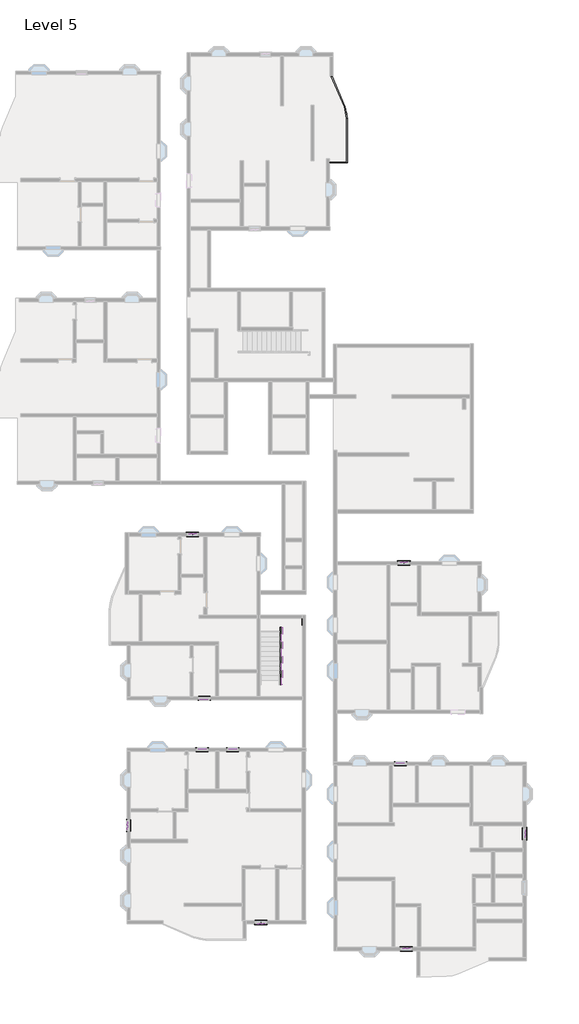
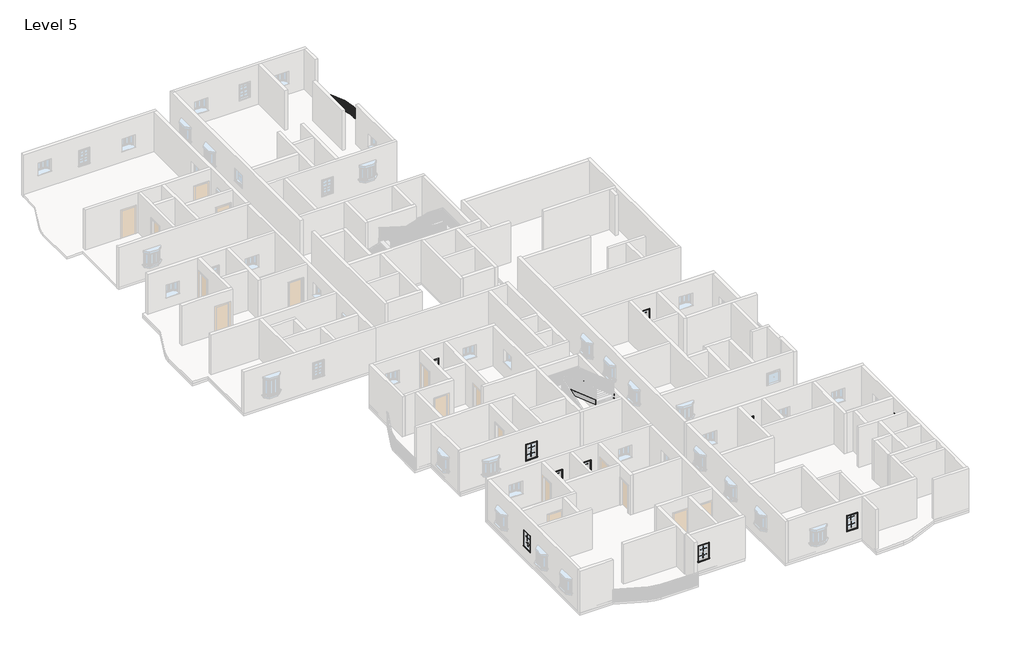
# One storey, part 13 of 14: 40 proxies, 6 members, 1 railing.
"""IFC4 building model written with IfcOpenShell, lengths in millimetres."""

from ifc_helpers import new_model, si_unit, frame, origin, place, context, project, spatial, polyline, circle_curve, outline, extrude, transform, mapped, element, save
from ifc_brep_helpers import plane_surface, cylinder_surface, revolved_surface, advanced_brep
from components import muntin_pattern_2x2_muntin_pattern_2x2_c35c595f, trim_window_exterior_flat_with_sill_e38017c9, trim_window_interior_flat_picture_frame_d728ed12

model = new_model("IFC4")

# Units and contexts
model_context = context("Model", 3, world=origin())
ifc_project = project(units=[si_unit("LENGTHUNIT", "METRE", prefix="MILLI")], contexts=[model_context])

# Site, building, storey
site = spatial("IfcSite", under=ifc_project)
building = spatial("IfcBuilding", under=site)
storey = spatial("IfcBuildingStorey", under=building, Name="Level 5", Elevation=12192.0)

# Proxies
placement = place(None, origin())
muntin_pattern_2x2_muntin_pattern_2x2_shape = muntin_pattern_2x2_muntin_pattern_2x2_c35c595f(model_context)
element("IfcBuildingElementProxy", 1, Name="Muntin Pattern_2x2 : Muntin Pattern_2x2", ObjectType="Muntin Pattern_2x2 : Muntin Pattern_2x2", at=placement, inside=storey, context=model_context, shape_type="MappedRepresentation", body=[
    mapped(muntin_pattern_2x2_muntin_pattern_2x2_shape, transform((-8150.287215, -357.5666506, 13662.025), x_axis=(1.0, 0.0, 0.0), y_axis=(0.0, 1.0, 0.0), z_axis=(0.0, 0.0, 1.0))),
])
element("IfcBuildingElementProxy", 2, Name="Muntin Pattern_2x2 : Muntin Pattern_2x2", ObjectType="Muntin Pattern_2x2 : Muntin Pattern_2x2", at=placement, inside=storey, context=model_context, shape_type="MappedRepresentation", body=[
    mapped(muntin_pattern_2x2_muntin_pattern_2x2_shape, transform((-8150.287215, -402.0166506, 13182.6), x_axis=(1.0, 0.0, 0.0), y_axis=(0.0, 1.0, 0.0), z_axis=(0.0, 0.0, 1.0))),
])
element("IfcBuildingElementProxy", 3, Name="Muntin Pattern_2x2 : Muntin Pattern_2x2", ObjectType="Muntin Pattern_2x2 : Muntin Pattern_2x2", at=placement, inside=storey, context=model_context, shape_type="MappedRepresentation", body=[
    mapped(muntin_pattern_2x2_muntin_pattern_2x2_shape, transform((-7397.812215, -10854.1166506, 13662.025), x_axis=(-1.0, 0.0, 0.0), y_axis=(0.0, -1.0, 0.0), z_axis=(0.0, 0.0, 1.0))),
])
element("IfcBuildingElementProxy", 4, Name="Muntin Pattern_2x2 : Muntin Pattern_2x2", ObjectType="Muntin Pattern_2x2 : Muntin Pattern_2x2", at=placement, inside=storey, context=model_context, shape_type="MappedRepresentation", body=[
    mapped(muntin_pattern_2x2_muntin_pattern_2x2_shape, transform((-7397.812215, -10809.6666506, 13182.6), x_axis=(-1.0, 0.0, 0.0), y_axis=(0.0, -1.0, 0.0), z_axis=(0.0, 0.0, 1.0))),
])
element("IfcBuildingElementProxy", 5, Name="Muntin Pattern_2x2 : Muntin Pattern_2x2", ObjectType="Muntin Pattern_2x2 : Muntin Pattern_2x2", at=placement, inside=storey, context=model_context, shape_type="MappedRepresentation", body=[
    mapped(muntin_pattern_2x2_muntin_pattern_2x2_shape, transform((-7540.687215, -13997.3666506, 13662.025), x_axis=(1.0, 0.0, 0.0), y_axis=(0.0, 1.0, 0.0), z_axis=(0.0, 0.0, 1.0))),
])
element("IfcBuildingElementProxy", 6, Name="Muntin Pattern_2x2 : Muntin Pattern_2x2", ObjectType="Muntin Pattern_2x2 : Muntin Pattern_2x2", at=placement, inside=storey, context=model_context, shape_type="MappedRepresentation", body=[
    mapped(muntin_pattern_2x2_muntin_pattern_2x2_shape, transform((-7540.687215, -14041.8166506, 13182.6), x_axis=(1.0, 0.0, 0.0), y_axis=(0.0, 1.0, 0.0), z_axis=(0.0, 0.0, 1.0))),
])
element("IfcBuildingElementProxy", 7, Name="Muntin Pattern_2x2 : Muntin Pattern_2x2", ObjectType="Muntin Pattern_2x2 : Muntin Pattern_2x2", at=placement, inside=storey, context=model_context, shape_type="MappedRepresentation", body=[
    mapped(muntin_pattern_2x2_muntin_pattern_2x2_shape, transform((-5597.587215, -13997.3666506, 13662.025), x_axis=(1.0, 0.0, 0.0), y_axis=(0.0, 1.0, 0.0), z_axis=(0.0, 0.0, 1.0))),
])
element("IfcBuildingElementProxy", 8, Name="Muntin Pattern_2x2 : Muntin Pattern_2x2", ObjectType="Muntin Pattern_2x2 : Muntin Pattern_2x2", at=placement, inside=storey, context=model_context, shape_type="MappedRepresentation", body=[
    mapped(muntin_pattern_2x2_muntin_pattern_2x2_shape, transform((-5597.587215, -14041.8166506, 13182.6), x_axis=(1.0, 0.0, 0.0), y_axis=(0.0, 1.0, 0.0), z_axis=(0.0, 0.0, 1.0))),
])
element("IfcBuildingElementProxy", 9, Name="Muntin Pattern_2x2 : Muntin Pattern_2x2", ObjectType="Muntin Pattern_2x2 : Muntin Pattern_2x2", at=placement, inside=storey, context=model_context, shape_type="MappedRepresentation", body=[
    mapped(muntin_pattern_2x2_muntin_pattern_2x2_shape, transform((-12255.562215, -18863.6994419, 13662.025), x_axis=(0.0, 1.0, 0.0), y_axis=(-1.0, 0.0, 0.0), z_axis=(0.0, 0.0, 1.0))),
])
element("IfcBuildingElementProxy", 10, Name="Muntin Pattern_2x2 : Muntin Pattern_2x2", ObjectType="Muntin Pattern_2x2 : Muntin Pattern_2x2", at=placement, inside=storey, context=model_context, shape_type="MappedRepresentation", body=[
    mapped(muntin_pattern_2x2_muntin_pattern_2x2_shape, transform((-12211.112215, -18863.6994419, 13182.6), x_axis=(0.0, 1.0, 0.0), y_axis=(-1.0, 0.0, 0.0), z_axis=(0.0, 0.0, 1.0))),
])
element("IfcBuildingElementProxy", 11, Name="Muntin Pattern_2x2 : Muntin Pattern_2x2", ObjectType="Muntin Pattern_2x2 : Muntin Pattern_2x2", at=placement, inside=storey, context=model_context, shape_type="MappedRepresentation", body=[
    mapped(muntin_pattern_2x2_muntin_pattern_2x2_shape, transform((-3806.2891351, -25065.4166506, 13662.025), x_axis=(-1.0, 0.0, 0.0), y_axis=(0.0, -1.0, 0.0), z_axis=(0.0, 0.0, 1.0))),
])
element("IfcBuildingElementProxy", 12, Name="Muntin Pattern_2x2 : Muntin Pattern_2x2", ObjectType="Muntin Pattern_2x2 : Muntin Pattern_2x2", at=placement, inside=storey, context=model_context, shape_type="MappedRepresentation", body=[
    mapped(muntin_pattern_2x2_muntin_pattern_2x2_shape, transform((-3806.2891351, -25020.9666506, 13182.6), x_axis=(-1.0, 0.0, 0.0), y_axis=(0.0, -1.0, 0.0), z_axis=(0.0, 0.0, 1.0))),
])
element("IfcBuildingElementProxy", 13, Name="Muntin Pattern_2x2 : Muntin Pattern_2x2", ObjectType="Muntin Pattern_2x2 : Muntin Pattern_2x2", at=placement, inside=storey, context=model_context, shape_type="MappedRepresentation", body=[
    mapped(muntin_pattern_2x2_muntin_pattern_2x2_shape, transform((5410.0380523, -26615.6292694, 13662.025), x_axis=(1.0, 0.0, 0.0), y_axis=(0.0, 1.0, 0.0), z_axis=(0.0, 0.0, 1.0))),
])
element("IfcBuildingElementProxy", 14, Name="Muntin Pattern_2x2 : Muntin Pattern_2x2", ObjectType="Muntin Pattern_2x2 : Muntin Pattern_2x2", at=placement, inside=storey, context=model_context, shape_type="MappedRepresentation", body=[
    mapped(muntin_pattern_2x2_muntin_pattern_2x2_shape, transform((5410.0380523, -26660.0792694, 13182.6), x_axis=(1.0, 0.0, 0.0), y_axis=(0.0, 1.0, 0.0), z_axis=(0.0, 0.0, 1.0))),
])
element("IfcBuildingElementProxy", 15, Name="Muntin Pattern_2x2 : Muntin Pattern_2x2", ObjectType="Muntin Pattern_2x2 : Muntin Pattern_2x2", at=placement, inside=storey, context=model_context, shape_type="MappedRepresentation", body=[
    mapped(muntin_pattern_2x2_muntin_pattern_2x2_shape, transform((12982.4130523, -19379.8042694, 13662.025), x_axis=(0.0, -1.0, 0.0), y_axis=(1.0, 0.0, 0.0), z_axis=(0.0, 0.0, 1.0))),
])
element("IfcBuildingElementProxy", 16, Name="Muntin Pattern_2x2 : Muntin Pattern_2x2", ObjectType="Muntin Pattern_2x2 : Muntin Pattern_2x2", at=placement, inside=storey, context=model_context, shape_type="MappedRepresentation", body=[
    mapped(muntin_pattern_2x2_muntin_pattern_2x2_shape, transform((12937.9630523, -19379.8042694, 13182.6), x_axis=(0.0, -1.0, 0.0), y_axis=(1.0, 0.0, 0.0), z_axis=(0.0, 0.0, 1.0))),
])
element("IfcBuildingElementProxy", 17, Name="Muntin Pattern_2x2 : Muntin Pattern_2x2", ObjectType="Muntin Pattern_2x2 : Muntin Pattern_2x2", at=placement, inside=storey, context=model_context, shape_type="MappedRepresentation", body=[
    mapped(muntin_pattern_2x2_muntin_pattern_2x2_shape, transform((5048.0880523, -14880.8292694, 13662.025), x_axis=(1.0, 0.0, 0.0), y_axis=(0.0, 1.0, 0.0), z_axis=(0.0, 0.0, 1.0))),
])
element("IfcBuildingElementProxy", 18, Name="Muntin Pattern_2x2 : Muntin Pattern_2x2", ObjectType="Muntin Pattern_2x2 : Muntin Pattern_2x2", at=placement, inside=storey, context=model_context, shape_type="MappedRepresentation", body=[
    mapped(muntin_pattern_2x2_muntin_pattern_2x2_shape, transform((5048.0880523, -14925.2792694, 13182.6), x_axis=(1.0, 0.0, 0.0), y_axis=(0.0, 1.0, 0.0), z_axis=(0.0, 0.0, 1.0))),
])
element("IfcBuildingElementProxy", 19, Name="Muntin Pattern_2x2 : Muntin Pattern_2x2", ObjectType="Muntin Pattern_2x2 : Muntin Pattern_2x2", at=placement, inside=storey, context=model_context, shape_type="MappedRepresentation", body=[
    mapped(muntin_pattern_2x2_muntin_pattern_2x2_shape, transform((5257.6380523, -2168.1292694, 13662.025), x_axis=(1.0, 0.0, 0.0), y_axis=(0.0, 1.0, 0.0), z_axis=(0.0, 0.0, 1.0))),
])
element("IfcBuildingElementProxy", 20, Name="Muntin Pattern_2x2 : Muntin Pattern_2x2", ObjectType="Muntin Pattern_2x2 : Muntin Pattern_2x2", at=placement, inside=storey, context=model_context, shape_type="MappedRepresentation", body=[
    mapped(muntin_pattern_2x2_muntin_pattern_2x2_shape, transform((5257.6380523, -2212.5792694, 13182.6), x_axis=(1.0, 0.0, 0.0), y_axis=(0.0, 1.0, 0.0), z_axis=(0.0, 0.0, 1.0))),
])
trim_window_exterior_flat_with_sill_shape = trim_window_exterior_flat_with_sill_e38017c9(model_context)
element("IfcBuildingElementProxy", 21, Name="Trim-Window-Exterior-Flat : with Sill", ObjectType="Trim-Window-Exterior-Flat : with Sill", at=placement, inside=storey, context=model_context, shape_type="MappedRepresentation", body=[
    mapped(trim_window_exterior_flat_with_sill_shape, transform((-8150.287215, -322.6416506, 14173.2), x_axis=(-1.0, 0.0, 0.0), y_axis=(0.0, 0.0, 1.0), z_axis=(0.0, 1.0, 0.0))),
])
element("IfcBuildingElementProxy", 22, Name="Trim-Window-Exterior-Flat : with Sill", ObjectType="Trim-Window-Exterior-Flat : with Sill", at=placement, inside=storey, context=model_context, shape_type="MappedRepresentation", body=[
    mapped(trim_window_exterior_flat_with_sill_shape, transform((-7397.812215, -10889.0416506, 14173.2), x_axis=(1.0, 0.0, 0.0), y_axis=(0.0, 0.0, 1.0), z_axis=(0.0, -1.0, 0.0))),
])
element("IfcBuildingElementProxy", 23, Name="Trim-Window-Exterior-Flat : with Sill", ObjectType="Trim-Window-Exterior-Flat : with Sill", at=placement, inside=storey, context=model_context, shape_type="MappedRepresentation", body=[
    mapped(trim_window_exterior_flat_with_sill_shape, transform((-7540.687215, -13962.4416506, 14173.2), x_axis=(-1.0, 0.0, 0.0), y_axis=(0.0, 0.0, 1.0), z_axis=(0.0, 1.0, 0.0))),
])
element("IfcBuildingElementProxy", 24, Name="Trim-Window-Exterior-Flat : with Sill", ObjectType="Trim-Window-Exterior-Flat : with Sill", at=placement, inside=storey, context=model_context, shape_type="MappedRepresentation", body=[
    mapped(trim_window_exterior_flat_with_sill_shape, transform((-5597.587215, -13962.4416506, 14173.2), x_axis=(-1.0, 0.0, 0.0), y_axis=(0.0, 0.0, 1.0), z_axis=(0.0, 1.0, 0.0))),
])
element("IfcBuildingElementProxy", 25, Name="Trim-Window-Exterior-Flat : with Sill", ObjectType="Trim-Window-Exterior-Flat : with Sill", at=placement, inside=storey, context=model_context, shape_type="MappedRepresentation", body=[
    mapped(trim_window_exterior_flat_with_sill_shape, transform((-12290.487215, -18863.6994419, 14173.2), x_axis=(0.0, -1.0, 0.0), y_axis=(0.0, 0.0, 1.0), z_axis=(-1.0, 0.0, 0.0))),
])
element("IfcBuildingElementProxy", 26, Name="Trim-Window-Exterior-Flat : with Sill", ObjectType="Trim-Window-Exterior-Flat : with Sill", at=placement, inside=storey, context=model_context, shape_type="MappedRepresentation", body=[
    mapped(trim_window_exterior_flat_with_sill_shape, transform((-3806.2891351, -25100.3416506, 14173.2), x_axis=(1.0, 0.0, 0.0), y_axis=(0.0, 0.0, 1.0), z_axis=(0.0, -1.0, 0.0))),
])
element("IfcBuildingElementProxy", 27, Name="Trim-Window-Exterior-Flat : with Sill", ObjectType="Trim-Window-Exterior-Flat : with Sill", at=placement, inside=storey, context=model_context, shape_type="MappedRepresentation", body=[
    mapped(trim_window_exterior_flat_with_sill_shape, transform((5410.0380523, -26580.7042694, 14173.2), x_axis=(-1.0, 0.0, 0.0), y_axis=(0.0, 0.0, 1.0), z_axis=(0.0, 1.0, 0.0))),
])
element("IfcBuildingElementProxy", 28, Name="Trim-Window-Exterior-Flat : with Sill", ObjectType="Trim-Window-Exterior-Flat : with Sill", at=placement, inside=storey, context=model_context, shape_type="MappedRepresentation", body=[
    mapped(trim_window_exterior_flat_with_sill_shape, transform((13017.3380523, -19379.8042694, 14173.2), x_axis=(0.0, 1.0, 0.0), y_axis=(0.0, 0.0, 1.0), z_axis=(1.0, 0.0, 0.0))),
])
element("IfcBuildingElementProxy", 29, Name="Trim-Window-Exterior-Flat : with Sill", ObjectType="Trim-Window-Exterior-Flat : with Sill", at=placement, inside=storey, context=model_context, shape_type="MappedRepresentation", body=[
    mapped(trim_window_exterior_flat_with_sill_shape, transform((5048.0880523, -14845.9042694, 14173.2), x_axis=(-1.0, 0.0, 0.0), y_axis=(0.0, 0.0, 1.0), z_axis=(0.0, 1.0, 0.0))),
])
element("IfcBuildingElementProxy", 30, Name="Trim-Window-Exterior-Flat : with Sill", ObjectType="Trim-Window-Exterior-Flat : with Sill", at=placement, inside=storey, context=model_context, shape_type="MappedRepresentation", body=[
    mapped(trim_window_exterior_flat_with_sill_shape, transform((5257.6380523, -2133.2042694, 14173.2), x_axis=(-1.0, 0.0, 0.0), y_axis=(0.0, 0.0, 1.0), z_axis=(0.0, 1.0, 0.0))),
])
trim_window_interior_flat_picture_frame_shape = trim_window_interior_flat_picture_frame_d728ed12(model_context)
element("IfcBuildingElementProxy", 31, Name="Trim-Window-Interior-Flat : Picture Frame", ObjectType="Trim-Window-Interior-Flat : Picture Frame", at=placement, inside=storey, context=model_context, shape_type="MappedRepresentation", body=[
    mapped(trim_window_interior_flat_picture_frame_shape, transform((-8150.287215, -525.8416506, 14173.2), x_axis=(1.0, 0.0, 0.0), y_axis=(0.0, 0.0, 1.0), z_axis=(0.0, -1.0, 0.0))),
])
element("IfcBuildingElementProxy", 32, Name="Trim-Window-Interior-Flat : Picture Frame", ObjectType="Trim-Window-Interior-Flat : Picture Frame", at=placement, inside=storey, context=model_context, shape_type="MappedRepresentation", body=[
    mapped(trim_window_interior_flat_picture_frame_shape, transform((-7397.812215, -10685.8416506, 14173.2), x_axis=(-1.0, 0.0, 0.0), y_axis=(0.0, 0.0, 1.0), z_axis=(0.0, 1.0, 0.0))),
])
element("IfcBuildingElementProxy", 33, Name="Trim-Window-Interior-Flat : Picture Frame", ObjectType="Trim-Window-Interior-Flat : Picture Frame", at=placement, inside=storey, context=model_context, shape_type="MappedRepresentation", body=[
    mapped(trim_window_interior_flat_picture_frame_shape, transform((-7540.687215, -14165.6416506, 14173.2), x_axis=(1.0, 0.0, 0.0), y_axis=(0.0, 0.0, 1.0), z_axis=(0.0, -1.0, 0.0))),
])
element("IfcBuildingElementProxy", 34, Name="Trim-Window-Interior-Flat : Picture Frame", ObjectType="Trim-Window-Interior-Flat : Picture Frame", at=placement, inside=storey, context=model_context, shape_type="MappedRepresentation", body=[
    mapped(trim_window_interior_flat_picture_frame_shape, transform((-5597.587215, -14165.6416506, 14173.2), x_axis=(1.0, 0.0, 0.0), y_axis=(0.0, 0.0, 1.0), z_axis=(0.0, -1.0, 0.0))),
])
element("IfcBuildingElementProxy", 35, Name="Trim-Window-Interior-Flat : Picture Frame", ObjectType="Trim-Window-Interior-Flat : Picture Frame", at=placement, inside=storey, context=model_context, shape_type="MappedRepresentation", body=[
    mapped(trim_window_interior_flat_picture_frame_shape, transform((-12087.287215, -18863.6994419, 14173.2), x_axis=(0.0, 1.0, 0.0), y_axis=(0.0, 0.0, 1.0), z_axis=(1.0, 0.0, 0.0))),
])
element("IfcBuildingElementProxy", 36, Name="Trim-Window-Interior-Flat : Picture Frame", ObjectType="Trim-Window-Interior-Flat : Picture Frame", at=placement, inside=storey, context=model_context, shape_type="MappedRepresentation", body=[
    mapped(trim_window_interior_flat_picture_frame_shape, transform((-3806.2891351, -24897.1416506, 14173.2), x_axis=(-1.0, 0.0, 0.0), y_axis=(0.0, 0.0, 1.0), z_axis=(0.0, 1.0, 0.0))),
])
element("IfcBuildingElementProxy", 37, Name="Trim-Window-Interior-Flat : Picture Frame", ObjectType="Trim-Window-Interior-Flat : Picture Frame", at=placement, inside=storey, context=model_context, shape_type="MappedRepresentation", body=[
    mapped(trim_window_interior_flat_picture_frame_shape, transform((5410.0380523, -26783.9042694, 14173.2), x_axis=(1.0, 0.0, 0.0), y_axis=(0.0, 0.0, 1.0), z_axis=(0.0, -1.0, 0.0))),
])
element("IfcBuildingElementProxy", 38, Name="Trim-Window-Interior-Flat : Picture Frame", ObjectType="Trim-Window-Interior-Flat : Picture Frame", at=placement, inside=storey, context=model_context, shape_type="MappedRepresentation", body=[
    mapped(trim_window_interior_flat_picture_frame_shape, transform((12814.1380523, -19379.8042694, 14173.2), x_axis=(0.0, -1.0, 0.0), y_axis=(0.0, 0.0, 1.0), z_axis=(-1.0, 0.0, 0.0))),
])
element("IfcBuildingElementProxy", 39, Name="Trim-Window-Interior-Flat : Picture Frame", ObjectType="Trim-Window-Interior-Flat : Picture Frame", at=placement, inside=storey, context=model_context, shape_type="MappedRepresentation", body=[
    mapped(trim_window_interior_flat_picture_frame_shape, transform((5048.0880523, -15049.1042694, 14173.2), x_axis=(1.0, 0.0, 0.0), y_axis=(0.0, 0.0, 1.0), z_axis=(0.0, -1.0, 0.0))),
])
element("IfcBuildingElementProxy", 40, Name="Trim-Window-Interior-Flat : Picture Frame", ObjectType="Trim-Window-Interior-Flat : Picture Frame", at=placement, inside=storey, context=model_context, shape_type="MappedRepresentation", body=[
    mapped(trim_window_interior_flat_picture_frame_shape, transform((5257.6380523, -2336.4042694, 14173.2), x_axis=(1.0, 0.0, 0.0), y_axis=(0.0, 0.0, 1.0), z_axis=(0.0, -1.0, 0.0))),
])

# Members
element("IfcMember", 41, ObjectType="Stringer - 2\" Width", at=placement, inside=storey, context=model_context, shape_type="SweptSolid", body=[
    extrude(outline(polyline([(-9955.5916506, 12192.0), (-9955.5916506, 12383.3592169), (-6325.8738327, 13639.8), (-5713.7916506, 13639.8), (-5713.7916506, 13529.1301656), (-9576.612129, 12192.0), (-9955.5916506, 12192.0)])), frame((-3908.487215, 0.0, 0.0), z_axis=(1.0, 0.0, 0.0), x_axis=(0.0, 1.0, 0.0)), (0.0, 0.0, 1.0), 50.8),
])
element("IfcMember", 42, ObjectType="Stringer - 2\" Width", at=placement, inside=storey, context=model_context, shape_type="SweptSolid", body=[
    extrude(outline(polyline([(-3908.487215, -5713.7916506), (-3908.487215, -5662.9916506), (-1190.687215, -5662.9916506), (-1190.687215, -5713.7916506), (-3908.487215, -5713.7916506)])), frame((0.0, 0.0, 13335.0), z_axis=(0.0, 0.0, 1.0), x_axis=(1.0, 0.0, 0.0)), (0.0, 0.0, 1.0), 304.8),
])
element("IfcMember", 43, ObjectType="Stringer - 2\" Width", at=placement, inside=storey, context=model_context, shape_type="SweptSolid", body=[
    extrude(outline(polyline([(-5662.9916506, 13539.5476784), (-5662.9916506, 13335.0), (-6003.8711722, 13335.0), (-9949.2416506, 14700.7051656), (-9949.2416506, 15023.2496015), (-5662.9916506, 13539.5476784)])), frame((-1190.687215, 0.0, 0.0), z_axis=(1.0, 0.0, 0.0), x_axis=(0.0, 1.0, 0.0)), (0.0, 0.0, 1.0), 50.8),
])
element("IfcMember", 44, ObjectType="Stringer - 2\" Width", at=placement, inside=storey, context=model_context, shape_type="SweptSolid", body=[
    extrude(outline(polyline([(-9955.5916506, 12192.0), (-9955.5916506, 12383.3592169), (-6342.4416506, 13634.0649861), (-6342.4416506, 13311.5205502), (-9576.612129, 12192.0), (-9955.5916506, 12192.0)])), frame((-2593.7381751, 0.0, 0.0), z_axis=(1.0, 0.0, 0.0), x_axis=(0.0, 1.0, 0.0)), (0.0, 0.0, 1.0), 50.8),
])
element("IfcMember", 45, ObjectType="Stringer - 2\" Width", at=placement, inside=storey, context=model_context, shape_type="SweptSolid", body=[
    extrude(outline(polyline([(-2593.7381751, -6342.4416506), (-2593.7381751, -6291.6416506), (-2492.1381751, -6291.6416506), (-2492.1381751, -6342.4416506), (-2593.7381751, -6342.4416506)])), frame((0.0, 0.0, 13335.0), z_axis=(0.0, 0.0, 1.0), x_axis=(1.0, 0.0, 0.0)), (0.0, 0.0, 1.0), 304.8),
])
element("IfcMember", 46, ObjectType="Stringer - 2\" Width", at=placement, inside=storey, context=model_context, shape_type="SweptSolid", body=[
    extrude(outline(polyline([(-6291.6416506, 13757.1572938), (-6291.6416506, 13434.6128579), (-9949.2416506, 14700.7051656), (-9949.2416506, 15023.2496015), (-6291.6416506, 13757.1572938)])), frame((-2492.1381751, 0.0, 0.0), z_axis=(1.0, 0.0, 0.0), x_axis=(0.0, 1.0, 0.0)), (0.0, 0.0, 1.0), 50.8),
])

# Railing
element("IfcRailing", 47, ObjectType="Handrail - Rectangular", at=placement, inside=storey, context=model_context, shape_type="SolidModel", body=[
    advanced_brep(
    [(549.8108649, 23180.4215905, 13106.4), (549.8108649, 23180.4215905, 13055.6), (549.8108649, 23129.6215905, 13055.6), (549.8108649, 23129.6215905, 13106.4), (1629.3108649, 23180.4215905, 13106.4), (1629.3108649, 23180.4215905, 13055.6), (1680.1108649, 23129.6215905, 13055.6), (1680.1108649, 23129.6215905, 13106.4), (1629.3108649, 25921.9580583, 13106.4), (1629.3108649, 25921.9580583, 13055.6), (1680.1108649, 25921.9580583, 13055.6), (1680.1108649, 25921.9580583, 13106.4), (1475.5051478, 26671.8537734, 13055.6), (1475.5051478, 26671.8537734, 13106.4), (1522.203662, 26691.8509925, 13055.6), (1522.203662, 26691.8509925, 13106.4), (640.7616078, 28621.188975, 13106.4), (687.460122, 28641.186194, 13106.4), (687.460122, 28641.186194, 13055.6), (640.7616078, 28621.188975, 13055.6)],
    [
        (0, 1),
        (1, 2),
        (2, 3),
        (3, 0),
        (0, 4),
        (4, 5),
        (5, 1),
        (5, 6),
        (6, 2),
        (6, 7),
        (7, 3),
        (7, 4),
        (4, 8),
        (8, 9),
        (9, 5),
        (9, 10),
        (10, 6),
        (10, 11),
        (11, 7),
        (11, 8),
        (12, 9, circle_curve(frame((-275.6891351, 25921.9580583, 13055.6), z_axis=(0.0, 0.0, -1.0), x_axis=(1.0, 0.0, 0.0)), 1905.0)),
        (8, 13, circle_curve(frame((-275.6891351, 25921.9580583, 13106.4), z_axis=(0.0, 0.0, 1.0), x_axis=(1.0, 0.0, 0.0)), 1905.0)),
        (13, 12),
        (14, 10, circle_curve(frame((-275.6891351, 25921.9580583, 13055.6), z_axis=(0.0, 0.0, -1.0), x_axis=(1.0, 0.0, 0.0)), 1955.8)),
        (12, 14),
        (15, 11, circle_curve(frame((-275.6891351, 25921.9580583, 13106.4), z_axis=(0.0, 0.0, -1.0), x_axis=(1.0, 0.0, 0.0)), 1955.8)),
        (14, 15),
        (15, 13),
        (16, 17),
        (17, 18),
        (18, 19),
        (19, 16),
        (13, 16),
        (19, 12),
        (18, 14),
        (17, 15),
    ],
    [
        plane_surface(frame((549.8108649, 23155.0215905, 13106.4), z_axis=(-1.0, 0.0, 0.0), x_axis=(0.0, 1.0, 0.0))),
        plane_surface(frame((549.8108649, 23180.4215905, 13106.4), z_axis=(0.0, 1.0, 0.0), x_axis=(1.0, 0.0, 0.0))),
        plane_surface(frame((549.8108649, 23180.4215905, 13055.6), z_axis=(0.0, 0.0, -1.0), x_axis=(1.0, 0.0, 0.0))),
        plane_surface(frame((549.8108649, 23129.6215905, 13055.6), z_axis=(0.0, -1.0, 0.0), x_axis=(1.0, 0.0, 0.0))),
        plane_surface(frame((549.8108649, 23129.6215905, 13106.4), z_axis=(0.0, 0.0, 1.0), x_axis=(1.0, 0.0, 0.0))),
        plane_surface(frame((1629.3108649, 23180.4215905, 13106.4), z_axis=(-1.0, 0.0, 0.0), x_axis=(0.0, 1.0, 0.0))),
        plane_surface(frame((1629.3108649, 23180.4215905, 13055.6), z_axis=(0.0, 0.0, -1.0), x_axis=(0.0, 1.0, 0.0))),
        plane_surface(frame((1680.1108649, 23129.6215905, 13055.6), z_axis=(1.0, 0.0, 0.0), x_axis=(0.0, 1.0, 0.0))),
        plane_surface(frame((1680.1108649, 23129.6215905, 13106.4), z_axis=(0.0, 0.0, 1.0), x_axis=(0.0, 1.0, 0.0))),
        revolved_surface(polyline([(1629.3108649, 25921.9580583, 13106.4), (1629.3108649, 25921.9580583, 13055.6)]), (-275.6891351, 25921.9580583, 13106.4), (0.0, 0.0, 1.0)),
        plane_surface(frame((-275.6891351, 25921.9580583, 13055.6), z_axis=(0.0, 0.0, -1.0), x_axis=(1.0, 0.0, 0.0))),
        cylinder_surface(frame((-275.6891351, 25921.9580583, 13106.4), z_axis=(0.0, 0.0, 1.0), x_axis=(1.0, 0.0, 0.0)), 1955.8),
        plane_surface(frame((-275.6891351, 25921.9580583, 13106.4), z_axis=(0.0, 0.0, 1.0), x_axis=(1.0, 0.0, 0.0))),
        plane_surface(frame((664.1108649, 28631.1875845, 13106.4), z_axis=(-0.39364604467361036, 0.91926209076238, 0.0), x_axis=(0.91926209076238, 0.39364604467361036, 0.0))),
        plane_surface(frame((1475.5051478, 26671.8537734, 13106.4), z_axis=(-0.91926209076238, -0.3936460446736102, 0.0), x_axis=(-0.3936460446736102, 0.91926209076238, 0.0))),
        plane_surface(frame((1475.5051478, 26671.8537734, 13055.6), z_axis=(0.0, 0.0, -1.0), x_axis=(-0.3936460446736102, 0.91926209076238, 0.0))),
        plane_surface(frame((1522.203662, 26691.8509925, 13055.6), z_axis=(0.91926209076238, 0.3936460446736102, 0.0), x_axis=(-0.3936460446736102, 0.91926209076238, 0.0))),
        plane_surface(frame((1522.203662, 26691.8509925, 13106.4), z_axis=(0.0, 0.0, 1.0), x_axis=(-0.3936460446736102, 0.91926209076238, 0.0))),
    ],
    [
        (0, [[1, 2, 3, 4]]),
        (1, [[-1, 5, 6, 7]]),
        (2, [[-2, -7, 8, 9]]),
        (3, [[-3, -9, 10, 11]]),
        (4, [[-4, -11, 12, -5]]),
        (5, [[-6, 13, 14, 15]]),
        (6, [[-8, -15, 16, 17]]),
        (7, [[-10, -17, 18, 19]]),
        (8, [[-12, -19, 20, -13]]),
        (9, [[21, -14, 22, 23]]),
        (10, [[24, -16, -21, 25]]),
        (11, [[26, -18, -24, 27]]),
        (12, [[-22, -20, -26, 28]]),
        (13, [[29, 30, 31, 32]]),
        (14, [[-23, 33, -32, 34]]),
        (15, [[-25, -34, -31, 35]]),
        (16, [[-27, -35, -30, 36]]),
        (17, [[-28, -36, -29, -33]]),
    ],
),
    extrude(outline(polyline([(711.4710921, 28544.7864585), (693.9591493, 28537.2875014), (686.4601921, 28554.7994442), (703.9721349, 28562.2984014), (711.4710921, 28544.7864585)])), frame((0.0, 0.0, 12192.0), z_axis=(0.0, 0.0, 1.0), x_axis=(1.0, 0.0, 0.0)), (0.0, 0.0, 1.0), 863.6),
    extrude(outline(polyline([(751.4655302, 28451.3894301), (733.9535874, 28443.890473), (726.4546303, 28461.4024158), (743.9665731, 28468.9013729), (751.4655302, 28451.3894301)])), frame((0.0, 0.0, 12192.0), z_axis=(0.0, 0.0, 1.0), x_axis=(1.0, 0.0, 0.0)), (0.0, 0.0, 1.0), 863.6),
    extrude(outline(polyline([(791.4599684, 28357.9924017), (773.9480255, 28350.4934445), (766.4490684, 28368.0053874), (783.9610112, 28375.5043445), (791.4599684, 28357.9924017)])), frame((0.0, 0.0, 12192.0), z_axis=(0.0, 0.0, 1.0), x_axis=(1.0, 0.0, 0.0)), (0.0, 0.0, 1.0), 863.6),
    extrude(outline(polyline([(831.4544065, 28264.5953733), (813.9424637, 28257.0964161), (806.4435065, 28274.608359), (823.9554494, 28282.1073161), (831.4544065, 28264.5953733)])), frame((0.0, 0.0, 12192.0), z_axis=(0.0, 0.0, 1.0), x_axis=(1.0, 0.0, 0.0)), (0.0, 0.0, 1.0), 863.6),
    extrude(outline(polyline([(871.4488446, 28171.1983449), (853.9369018, 28163.6993877), (846.4379447, 28181.2113305), (863.9498875, 28188.7102877), (871.4488446, 28171.1983449)])), frame((0.0, 0.0, 12192.0), z_axis=(0.0, 0.0, 1.0), x_axis=(1.0, 0.0, 0.0)), (0.0, 0.0, 1.0), 863.6),
    extrude(outline(polyline([(911.4432828, 28077.8013164), (893.93134, 28070.3023593), (886.4323828, 28087.8143021), (903.9443256, 28095.3132593), (911.4432828, 28077.8013164)])), frame((0.0, 0.0, 12192.0), z_axis=(0.0, 0.0, 1.0), x_axis=(1.0, 0.0, 0.0)), (0.0, 0.0, 1.0), 863.6),
    extrude(outline(polyline([(951.4377209, 27984.404288), (933.9257781, 27976.9053309), (926.4268209, 27994.4172737), (943.9387638, 28001.9162308), (951.4377209, 27984.404288)])), frame((0.0, 0.0, 12192.0), z_axis=(0.0, 0.0, 1.0), x_axis=(1.0, 0.0, 0.0)), (0.0, 0.0, 1.0), 863.6),
    extrude(outline(polyline([(991.4321591, 27891.0072596), (973.9202162, 27883.5083024), (966.4212591, 27901.0202453), (983.9332019, 27908.5192024), (991.4321591, 27891.0072596)])), frame((0.0, 0.0, 12192.0), z_axis=(0.0, 0.0, 1.0), x_axis=(1.0, 0.0, 0.0)), (0.0, 0.0, 1.0), 863.6),
    extrude(outline(polyline([(1031.4265972, 27797.6102312), (1013.9146544, 27790.111274), (1006.4156972, 27807.6232168), (1023.9276401, 27815.122174), (1031.4265972, 27797.6102312)])), frame((0.0, 0.0, 12192.0), z_axis=(0.0, 0.0, 1.0), x_axis=(1.0, 0.0, 0.0)), (0.0, 0.0, 1.0), 863.6),
    extrude(outline(polyline([(1071.4210353, 27704.2132027), (1053.9090925, 27696.7142456), (1046.4101354, 27714.2261884), (1063.9220782, 27721.7251456), (1071.4210353, 27704.2132027)])), frame((0.0, 0.0, 12192.0), z_axis=(0.0, 0.0, 1.0), x_axis=(1.0, 0.0, 0.0)), (0.0, 0.0, 1.0), 863.6),
    extrude(outline(polyline([(1111.4154735, 27610.8161743), (1093.9035307, 27603.3172172), (1086.4045735, 27620.82916), (1103.9165163, 27628.3281172), (1111.4154735, 27610.8161743)])), frame((0.0, 0.0, 12192.0), z_axis=(0.0, 0.0, 1.0), x_axis=(1.0, 0.0, 0.0)), (0.0, 0.0, 1.0), 863.6),
    extrude(outline(polyline([(1151.4099116, 27517.4191459), (1133.8979688, 27509.9201888), (1126.3990116, 27527.4321316), (1143.9109545, 27534.9310887), (1151.4099116, 27517.4191459)])), frame((0.0, 0.0, 12192.0), z_axis=(0.0, 0.0, 1.0), x_axis=(1.0, 0.0, 0.0)), (0.0, 0.0, 1.0), 863.6),
    extrude(outline(polyline([(1191.4043498, 27424.0221175), (1173.8924069, 27416.5231603), (1166.3934498, 27434.0351032), (1183.9053926, 27441.5340603), (1191.4043498, 27424.0221175)])), frame((0.0, 0.0, 12192.0), z_axis=(0.0, 0.0, 1.0), x_axis=(1.0, 0.0, 0.0)), (0.0, 0.0, 1.0), 863.6),
    extrude(outline(polyline([(1231.3987879, 27330.6250891), (1213.8868451, 27323.1261319), (1206.3878879, 27340.6380747), (1223.8998307, 27348.1370319), (1231.3987879, 27330.6250891)])), frame((0.0, 0.0, 12192.0), z_axis=(0.0, 0.0, 1.0), x_axis=(1.0, 0.0, 0.0)), (0.0, 0.0, 1.0), 863.6),
    extrude(outline(polyline([(1271.393226, 27237.2280606), (1253.8812832, 27229.7291035), (1246.3823261, 27247.2410463), (1263.8942689, 27254.7400035), (1271.393226, 27237.2280606)])), frame((0.0, 0.0, 12192.0), z_axis=(0.0, 0.0, 1.0), x_axis=(1.0, 0.0, 0.0)), (0.0, 0.0, 1.0), 863.6),
    extrude(outline(polyline([(1311.3876642, 27143.8310322), (1293.8757213, 27136.3320751), (1286.3767642, 27153.8440179), (1303.888707, 27161.342975), (1311.3876642, 27143.8310322)])), frame((0.0, 0.0, 12192.0), z_axis=(0.0, 0.0, 1.0), x_axis=(1.0, 0.0, 0.0)), (0.0, 0.0, 1.0), 863.6),
    extrude(outline(polyline([(1351.3821023, 27050.4340038), (1333.8701595, 27042.9350466), (1326.3712023, 27060.4469895), (1343.8831452, 27067.9459466), (1351.3821023, 27050.4340038)])), frame((0.0, 0.0, 12192.0), z_axis=(0.0, 0.0, 1.0), x_axis=(1.0, 0.0, 0.0)), (0.0, 0.0, 1.0), 863.6),
    extrude(outline(polyline([(1391.3765405, 26957.0369754), (1373.8645976, 26949.5380182), (1366.3656405, 26967.0499611), (1383.8775833, 26974.5489182), (1391.3765405, 26957.0369754)])), frame((0.0, 0.0, 12192.0), z_axis=(0.0, 0.0, 1.0), x_axis=(1.0, 0.0, 0.0)), (0.0, 0.0, 1.0), 863.6),
    extrude(outline(polyline([(1431.3709786, 26863.639947), (1413.8590358, 26856.1409898), (1406.3600786, 26873.6529326), (1423.8720214, 26881.1518898), (1431.3709786, 26863.639947)])), frame((0.0, 0.0, 12192.0), z_axis=(0.0, 0.0, 1.0), x_axis=(1.0, 0.0, 0.0)), (0.0, 0.0, 1.0), 863.6),
    extrude(outline(polyline([(1471.3654167, 26770.2429185), (1453.8534739, 26762.7439614), (1446.3545168, 26780.2559042), (1463.8664596, 26787.7548614), (1471.3654167, 26770.2429185)])), frame((0.0, 0.0, 12192.0), z_axis=(0.0, 0.0, 1.0), x_axis=(1.0, 0.0, 0.0)), (0.0, 0.0, 1.0), 863.6),
    extrude(outline(polyline([(1537.4917391, 26611.722401), (1519.7200483, 26604.8616791), (1512.8593263, 26622.6333699), (1530.6310171, 26629.4940918), (1537.4917391, 26611.722401)])), frame((0.0, 0.0, 12192.0), z_axis=(0.0, 0.0, 1.0), x_axis=(1.0, 0.0, 0.0)), (0.0, 0.0, 1.0), 863.6),
    extrude(outline(polyline([(1571.2676162, 26515.3807493), (1553.1596103, 26509.4644479), (1547.2433088, 26527.5724538), (1565.3513147, 26533.4887552), (1571.2676162, 26515.3807493)])), frame((0.0, 0.0, 12192.0), z_axis=(0.0, 0.0, 1.0), x_axis=(1.0, 0.0, 0.0)), (0.0, 0.0, 1.0), 863.6),
    extrude(outline(polyline([(1599.9284504, 26417.3956468), (1581.5342785, 26412.4401508), (1576.5787825, 26430.8343227), (1594.9729544, 26435.7898187), (1599.9284504, 26417.3956468)])), frame((0.0, 0.0, 12192.0), z_axis=(0.0, 0.0, 1.0), x_axis=(1.0, 0.0, 0.0)), (0.0, 0.0, 1.0), 863.6),
    extrude(outline(polyline([(1623.3948673, 26318.0384578), (1604.7654711, 26314.0574912), (1600.7845045, 26332.6868874), (1619.4139008, 26336.667854), (1623.3948673, 26318.0384578)])), frame((0.0, 0.0, 12192.0), z_axis=(0.0, 0.0, 1.0), x_axis=(1.0, 0.0, 0.0)), (0.0, 0.0, 1.0), 863.6),
    extrude(outline(polyline([(1641.601878, 26217.5843464), (1622.7888504, 26214.5889343), (1619.7934383, 26233.4019618), (1638.6064659, 26236.3973739), (1641.601878, 26217.5843464)])), frame((0.0, 0.0, 12192.0), z_axis=(0.0, 0.0, 1.0), x_axis=(1.0, 0.0, 0.0)), (0.0, 0.0, 1.0), 863.6),
    extrude(outline(polyline([(1654.4990591, 26116.3115146), (1635.5545019, 26114.3099526), (1633.5529398, 26133.2545098), (1652.4974971, 26135.2560719), (1654.4990591, 26116.3115146)])), frame((0.0, 0.0, 12192.0), z_axis=(0.0, 0.0, 1.0), x_axis=(1.0, 0.0, 0.0)), (0.0, 0.0, 1.0), 863.6),
    extrude(outline(polyline([(1662.0506927, 26014.5004319), (1643.0270716, 26013.4982632), (1642.0249029, 26032.5218842), (1661.048524, 26033.524053), (1662.0506927, 26014.5004319)])), frame((0.0, 0.0, 12192.0), z_axis=(0.0, 0.0, 1.0), x_axis=(1.0, 0.0, 0.0)), (0.0, 0.0, 1.0), 863.6),
    extrude(outline(polyline([(1664.2358649, 25888.6965905), (1645.1858649, 25888.6965905), (1645.1858649, 25907.7465905), (1664.2358649, 25907.7465905), (1664.2358649, 25888.6965905)])), frame((0.0, 0.0, 12192.0), z_axis=(0.0, 0.0, 1.0), x_axis=(1.0, 0.0, 0.0)), (0.0, 0.0, 1.0), 863.6),
    extrude(outline(polyline([(1664.2358649, 25787.0965905), (1645.1858649, 25787.0965905), (1645.1858649, 25806.1465905), (1664.2358649, 25806.1465905), (1664.2358649, 25787.0965905)])), frame((0.0, 0.0, 12192.0), z_axis=(0.0, 0.0, 1.0), x_axis=(1.0, 0.0, 0.0)), (0.0, 0.0, 1.0), 863.6),
    extrude(outline(polyline([(1664.2358649, 25685.4965905), (1645.1858649, 25685.4965905), (1645.1858649, 25704.5465905), (1664.2358649, 25704.5465905), (1664.2358649, 25685.4965905)])), frame((0.0, 0.0, 12192.0), z_axis=(0.0, 0.0, 1.0), x_axis=(1.0, 0.0, 0.0)), (0.0, 0.0, 1.0), 863.6),
    extrude(outline(polyline([(1664.2358649, 25583.8965905), (1645.1858649, 25583.8965905), (1645.1858649, 25602.9465905), (1664.2358649, 25602.9465905), (1664.2358649, 25583.8965905)])), frame((0.0, 0.0, 12192.0), z_axis=(0.0, 0.0, 1.0), x_axis=(1.0, 0.0, 0.0)), (0.0, 0.0, 1.0), 863.6),
    extrude(outline(polyline([(1664.2358649, 25482.2965905), (1645.1858649, 25482.2965905), (1645.1858649, 25501.3465905), (1664.2358649, 25501.3465905), (1664.2358649, 25482.2965905)])), frame((0.0, 0.0, 12192.0), z_axis=(0.0, 0.0, 1.0), x_axis=(1.0, 0.0, 0.0)), (0.0, 0.0, 1.0), 863.6),
    extrude(outline(polyline([(1664.2358649, 25380.6965905), (1645.1858649, 25380.6965905), (1645.1858649, 25399.7465905), (1664.2358649, 25399.7465905), (1664.2358649, 25380.6965905)])), frame((0.0, 0.0, 12192.0), z_axis=(0.0, 0.0, 1.0), x_axis=(1.0, 0.0, 0.0)), (0.0, 0.0, 1.0), 863.6),
    extrude(outline(polyline([(1664.2358649, 25279.0965905), (1645.1858649, 25279.0965905), (1645.1858649, 25298.1465905), (1664.2358649, 25298.1465905), (1664.2358649, 25279.0965905)])), frame((0.0, 0.0, 12192.0), z_axis=(0.0, 0.0, 1.0), x_axis=(1.0, 0.0, 0.0)), (0.0, 0.0, 1.0), 863.6),
    extrude(outline(polyline([(1664.2358649, 25177.4965905), (1645.1858649, 25177.4965905), (1645.1858649, 25196.5465905), (1664.2358649, 25196.5465905), (1664.2358649, 25177.4965905)])), frame((0.0, 0.0, 12192.0), z_axis=(0.0, 0.0, 1.0), x_axis=(1.0, 0.0, 0.0)), (0.0, 0.0, 1.0), 863.6),
    extrude(outline(polyline([(1664.2358649, 25075.8965905), (1645.1858649, 25075.8965905), (1645.1858649, 25094.9465905), (1664.2358649, 25094.9465905), (1664.2358649, 25075.8965905)])), frame((0.0, 0.0, 12192.0), z_axis=(0.0, 0.0, 1.0), x_axis=(1.0, 0.0, 0.0)), (0.0, 0.0, 1.0), 863.6),
    extrude(outline(polyline([(1664.2358649, 24974.2965905), (1645.1858649, 24974.2965905), (1645.1858649, 24993.3465905), (1664.2358649, 24993.3465905), (1664.2358649, 24974.2965905)])), frame((0.0, 0.0, 12192.0), z_axis=(0.0, 0.0, 1.0), x_axis=(1.0, 0.0, 0.0)), (0.0, 0.0, 1.0), 863.6),
    extrude(outline(polyline([(1664.2358649, 24872.6965905), (1645.1858649, 24872.6965905), (1645.1858649, 24891.7465905), (1664.2358649, 24891.7465905), (1664.2358649, 24872.6965905)])), frame((0.0, 0.0, 12192.0), z_axis=(0.0, 0.0, 1.0), x_axis=(1.0, 0.0, 0.0)), (0.0, 0.0, 1.0), 863.6),
    extrude(outline(polyline([(1664.2358649, 24771.0965905), (1645.1858649, 24771.0965905), (1645.1858649, 24790.1465905), (1664.2358649, 24790.1465905), (1664.2358649, 24771.0965905)])), frame((0.0, 0.0, 12192.0), z_axis=(0.0, 0.0, 1.0), x_axis=(1.0, 0.0, 0.0)), (0.0, 0.0, 1.0), 863.6),
    extrude(outline(polyline([(1664.2358649, 24669.4965905), (1645.1858649, 24669.4965905), (1645.1858649, 24688.5465905), (1664.2358649, 24688.5465905), (1664.2358649, 24669.4965905)])), frame((0.0, 0.0, 12192.0), z_axis=(0.0, 0.0, 1.0), x_axis=(1.0, 0.0, 0.0)), (0.0, 0.0, 1.0), 863.6),
    extrude(outline(polyline([(1664.2358649, 24567.8965905), (1645.1858649, 24567.8965905), (1645.1858649, 24586.9465905), (1664.2358649, 24586.9465905), (1664.2358649, 24567.8965905)])), frame((0.0, 0.0, 12192.0), z_axis=(0.0, 0.0, 1.0), x_axis=(1.0, 0.0, 0.0)), (0.0, 0.0, 1.0), 863.6),
    extrude(outline(polyline([(1664.2358649, 24466.2965905), (1645.1858649, 24466.2965905), (1645.1858649, 24485.3465905), (1664.2358649, 24485.3465905), (1664.2358649, 24466.2965905)])), frame((0.0, 0.0, 12192.0), z_axis=(0.0, 0.0, 1.0), x_axis=(1.0, 0.0, 0.0)), (0.0, 0.0, 1.0), 863.6),
    extrude(outline(polyline([(1664.2358649, 24364.6965905), (1645.1858649, 24364.6965905), (1645.1858649, 24383.7465905), (1664.2358649, 24383.7465905), (1664.2358649, 24364.6965905)])), frame((0.0, 0.0, 12192.0), z_axis=(0.0, 0.0, 1.0), x_axis=(1.0, 0.0, 0.0)), (0.0, 0.0, 1.0), 863.6),
    extrude(outline(polyline([(1664.2358649, 24263.0965905), (1645.1858649, 24263.0965905), (1645.1858649, 24282.1465905), (1664.2358649, 24282.1465905), (1664.2358649, 24263.0965905)])), frame((0.0, 0.0, 12192.0), z_axis=(0.0, 0.0, 1.0), x_axis=(1.0, 0.0, 0.0)), (0.0, 0.0, 1.0), 863.6),
    extrude(outline(polyline([(1664.2358649, 24161.4965905), (1645.1858649, 24161.4965905), (1645.1858649, 24180.5465905), (1664.2358649, 24180.5465905), (1664.2358649, 24161.4965905)])), frame((0.0, 0.0, 12192.0), z_axis=(0.0, 0.0, 1.0), x_axis=(1.0, 0.0, 0.0)), (0.0, 0.0, 1.0), 863.6),
    extrude(outline(polyline([(1664.2358649, 24059.8965905), (1645.1858649, 24059.8965905), (1645.1858649, 24078.9465905), (1664.2358649, 24078.9465905), (1664.2358649, 24059.8965905)])), frame((0.0, 0.0, 12192.0), z_axis=(0.0, 0.0, 1.0), x_axis=(1.0, 0.0, 0.0)), (0.0, 0.0, 1.0), 863.6),
    extrude(outline(polyline([(1664.2358649, 23958.2965905), (1645.1858649, 23958.2965905), (1645.1858649, 23977.3465905), (1664.2358649, 23977.3465905), (1664.2358649, 23958.2965905)])), frame((0.0, 0.0, 12192.0), z_axis=(0.0, 0.0, 1.0), x_axis=(1.0, 0.0, 0.0)), (0.0, 0.0, 1.0), 863.6),
    extrude(outline(polyline([(1664.2358649, 23856.6965905), (1645.1858649, 23856.6965905), (1645.1858649, 23875.7465905), (1664.2358649, 23875.7465905), (1664.2358649, 23856.6965905)])), frame((0.0, 0.0, 12192.0), z_axis=(0.0, 0.0, 1.0), x_axis=(1.0, 0.0, 0.0)), (0.0, 0.0, 1.0), 863.6),
    extrude(outline(polyline([(1664.2358649, 23755.0965905), (1645.1858649, 23755.0965905), (1645.1858649, 23774.1465905), (1664.2358649, 23774.1465905), (1664.2358649, 23755.0965905)])), frame((0.0, 0.0, 12192.0), z_axis=(0.0, 0.0, 1.0), x_axis=(1.0, 0.0, 0.0)), (0.0, 0.0, 1.0), 863.6),
    extrude(outline(polyline([(1664.2358649, 23653.4965905), (1645.1858649, 23653.4965905), (1645.1858649, 23672.5465905), (1664.2358649, 23672.5465905), (1664.2358649, 23653.4965905)])), frame((0.0, 0.0, 12192.0), z_axis=(0.0, 0.0, 1.0), x_axis=(1.0, 0.0, 0.0)), (0.0, 0.0, 1.0), 863.6),
    extrude(outline(polyline([(1664.2358649, 23551.8965905), (1645.1858649, 23551.8965905), (1645.1858649, 23570.9465905), (1664.2358649, 23570.9465905), (1664.2358649, 23551.8965905)])), frame((0.0, 0.0, 12192.0), z_axis=(0.0, 0.0, 1.0), x_axis=(1.0, 0.0, 0.0)), (0.0, 0.0, 1.0), 863.6),
    extrude(outline(polyline([(1664.2358649, 23450.2965905), (1645.1858649, 23450.2965905), (1645.1858649, 23469.3465905), (1664.2358649, 23469.3465905), (1664.2358649, 23450.2965905)])), frame((0.0, 0.0, 12192.0), z_axis=(0.0, 0.0, 1.0), x_axis=(1.0, 0.0, 0.0)), (0.0, 0.0, 1.0), 863.6),
    extrude(outline(polyline([(1664.2358649, 23348.6965905), (1645.1858649, 23348.6965905), (1645.1858649, 23367.7465905), (1664.2358649, 23367.7465905), (1664.2358649, 23348.6965905)])), frame((0.0, 0.0, 12192.0), z_axis=(0.0, 0.0, 1.0), x_axis=(1.0, 0.0, 0.0)), (0.0, 0.0, 1.0), 863.6),
    extrude(outline(polyline([(1664.2358649, 23247.0965905), (1645.1858649, 23247.0965905), (1645.1858649, 23266.1465905), (1664.2358649, 23266.1465905), (1664.2358649, 23247.0965905)])), frame((0.0, 0.0, 12192.0), z_axis=(0.0, 0.0, 1.0), x_axis=(1.0, 0.0, 0.0)), (0.0, 0.0, 1.0), 863.6),
    extrude(outline(polyline([(1556.2858649, 23145.4965905), (1556.2858649, 23164.5465905), (1575.3358649, 23164.5465905), (1575.3358649, 23145.4965905), (1556.2858649, 23145.4965905)])), frame((0.0, 0.0, 12192.0), z_axis=(0.0, 0.0, 1.0), x_axis=(1.0, 0.0, 0.0)), (0.0, 0.0, 1.0), 863.6),
    extrude(outline(polyline([(1454.6858649, 23145.4965905), (1454.6858649, 23164.5465905), (1473.7358649, 23164.5465905), (1473.7358649, 23145.4965905), (1454.6858649, 23145.4965905)])), frame((0.0, 0.0, 12192.0), z_axis=(0.0, 0.0, 1.0), x_axis=(1.0, 0.0, 0.0)), (0.0, 0.0, 1.0), 863.6),
    extrude(outline(polyline([(1353.0858649, 23145.4965905), (1353.0858649, 23164.5465905), (1372.1358649, 23164.5465905), (1372.1358649, 23145.4965905), (1353.0858649, 23145.4965905)])), frame((0.0, 0.0, 12192.0), z_axis=(0.0, 0.0, 1.0), x_axis=(1.0, 0.0, 0.0)), (0.0, 0.0, 1.0), 863.6),
    extrude(outline(polyline([(1251.4858649, 23145.4965905), (1251.4858649, 23164.5465905), (1270.5358649, 23164.5465905), (1270.5358649, 23145.4965905), (1251.4858649, 23145.4965905)])), frame((0.0, 0.0, 12192.0), z_axis=(0.0, 0.0, 1.0), x_axis=(1.0, 0.0, 0.0)), (0.0, 0.0, 1.0), 863.6),
    extrude(outline(polyline([(1149.8858649, 23145.4965905), (1149.8858649, 23164.5465905), (1168.9358649, 23164.5465905), (1168.9358649, 23145.4965905), (1149.8858649, 23145.4965905)])), frame((0.0, 0.0, 12192.0), z_axis=(0.0, 0.0, 1.0), x_axis=(1.0, 0.0, 0.0)), (0.0, 0.0, 1.0), 863.6),
    extrude(outline(polyline([(1048.2858649, 23145.4965905), (1048.2858649, 23164.5465905), (1067.3358649, 23164.5465905), (1067.3358649, 23145.4965905), (1048.2858649, 23145.4965905)])), frame((0.0, 0.0, 12192.0), z_axis=(0.0, 0.0, 1.0), x_axis=(1.0, 0.0, 0.0)), (0.0, 0.0, 1.0), 863.6),
    extrude(outline(polyline([(946.6858649, 23145.4965905), (946.6858649, 23164.5465905), (965.7358649, 23164.5465905), (965.7358649, 23145.4965905), (946.6858649, 23145.4965905)])), frame((0.0, 0.0, 12192.0), z_axis=(0.0, 0.0, 1.0), x_axis=(1.0, 0.0, 0.0)), (0.0, 0.0, 1.0), 863.6),
    extrude(outline(polyline([(845.0858649, 23145.4965905), (845.0858649, 23164.5465905), (864.1358649, 23164.5465905), (864.1358649, 23145.4965905), (845.0858649, 23145.4965905)])), frame((0.0, 0.0, 12192.0), z_axis=(0.0, 0.0, 1.0), x_axis=(1.0, 0.0, 0.0)), (0.0, 0.0, 1.0), 863.6),
    extrude(outline(polyline([(743.4858649, 23145.4965905), (743.4858649, 23164.5465905), (762.5358649, 23164.5465905), (762.5358649, 23145.4965905), (743.4858649, 23145.4965905)])), frame((0.0, 0.0, 12192.0), z_axis=(0.0, 0.0, 1.0), x_axis=(1.0, 0.0, 0.0)), (0.0, 0.0, 1.0), 863.6),
    extrude(outline(polyline([(641.8858649, 23145.4965905), (641.8858649, 23164.5465905), (660.9358649, 23164.5465905), (660.9358649, 23145.4965905), (641.8858649, 23145.4965905)])), frame((0.0, 0.0, 12192.0), z_axis=(0.0, 0.0, 1.0), x_axis=(1.0, 0.0, 0.0)), (0.0, 0.0, 1.0), 863.6),
    extrude(outline(polyline([(1511.3598549, 26676.8458901), (1493.847912, 26669.346933), (1486.3489549, 26686.8588758), (1503.8608977, 26694.3578329), (1511.3598549, 26676.8458901)])), frame((0.0, 0.0, 12192.0), z_axis=(0.0, 0.0, 1.0), x_axis=(1.0, 0.0, 0.0)), (0.0, 0.0, 1.0), 863.6),
    extrude(outline(polyline([(1664.2358649, 25912.4330583), (1645.1858649, 25912.4330583), (1645.1858649, 25931.4830583), (1664.2358649, 25931.4830583), (1664.2358649, 25912.4330583)])), frame((0.0, 0.0, 12192.0), z_axis=(0.0, 0.0, 1.0), x_axis=(1.0, 0.0, 0.0)), (0.0, 0.0, 1.0), 863.6),
    extrude(outline(polyline([(1645.1858649, 23145.4965905), (1645.1858649, 23164.5465905), (1664.2358649, 23164.5465905), (1664.2358649, 23145.4965905), (1645.1858649, 23145.4965905)])), frame((0.0, 0.0, 12192.0), z_axis=(0.0, 0.0, 1.0), x_axis=(1.0, 0.0, 0.0)), (0.0, 0.0, 1.0), 863.6),
    extrude(outline(polyline([(680.3657934, 28617.4251203), (662.8538506, 28609.9261631), (655.3548935, 28627.4381059), (672.8668363, 28634.9370631), (680.3657934, 28617.4251203)])), frame((0.0, 0.0, 12192.0), z_axis=(0.0, 0.0, 1.0), x_axis=(1.0, 0.0, 0.0)), (0.0, 0.0, 1.0), 863.6),
    extrude(outline(polyline([(549.8108649, 23145.4965905), (549.8108649, 23164.5465905), (568.8608649, 23164.5465905), (568.8608649, 23145.4965905), (549.8108649, 23145.4965905)])), frame((0.0, 0.0, 12192.0), z_axis=(0.0, 0.0, 1.0), x_axis=(1.0, 0.0, 0.0)), (0.0, 0.0, 1.0), 863.6),
])

save(model, "model.ifc")

# Revit data of these elements
# Type "Muntin Pattern_2x2 : Muntin Pattern_2x2"
#   Width [instance default] = 4' - 0"
#   Thickness = 0' - 0 1/2"
#   Height [instance default] = 4' - 0"
#   Distance = 0' - 0 3/4"
#   Interior Material [instance default] = none
#   Exterior Material [instance default] = none
#   Default Elevation = 0
# Type "Trim-Window-Exterior-Flat : with Sill"
#   Trim Width = 0' - 2 1/4"
#   Trim Thickness_Picture Frame = 0' - 1 1/4"
#   Trim Thickness_with Sill = 0' - 0 3/4"
#   Sill Thickness = 0' - 1 1/4"
#   Opening Width [instance default] = 2' - 0"
#   Opening Height [instance default] = 3' - 0"
#   Default Elevation = 4' - 0"
#   Sill = yes
#   Picture Frame = no
#   Trim Material [instance default] = none
# Type "Trim-Window-Interior-Flat : Picture Frame"
#   Trim Thickness_Picture Frame = 0' - 1 1/4"
#   Trim Width = 0' - 2 1/4"
#   Trim Thickness_with Sill = 0' - 0 3/4"
#   Sill Thickness = 0' - 1 1/4"
#   Opening Width [instance default] = 2' - 0"
#   Opening Height [instance default] = 3' - 0"
#   Default Elevation = 4' - 0"
#   Sill = no
#   Picture Frame = yes
#   Trim Material [instance default] = none
# Type "Handrail - Rectangular"
#   Assembly Code = "C2010400"
#   built-in parameter 1008612 = 0.0416667 (stored number, unit not read)
#   built-in parameter 1008611 = 0.0416667 (stored number, unit not read)
#   built-in parameter 1008609 = 0.333333 (stored number, unit not read)
#   built-in parameter 1008604 = 0.166667 (stored number, unit not read)
#   built-in parameter 1008603 = 0.166667 (stored number, unit not read)
#   Railing Height = 3' - 0"
#   built-in parameter 1008630 = 2
#   built-in parameter 1008610 = 2
#   built-in parameter 1008618 = Baluster - Square : 3/4"
# Elements 1, 2, 3, 4, 5, 6, 7, 8, 9, 10, 11, 12, 13, 14, 15, 16, 17, 18, 19, 20 (IfcBuildingElementProxy, "Muntin Pattern_2x2 : Muntin Pattern_2x2")
#   Width = 1' - 8"
#   Height = 1' - 5 1/8"
#   Interior Material = Wood - Stained
#   Exterior Material = Clad - White
#   Phase Created = New Construction
#   Materials on its faces: "Clad - White", "Wood - Stained"
# Elements 21, 22, 23, 24, 25, 26, 27, 28, 29, 30 (IfcBuildingElementProxy, "Trim-Window-Exterior-Flat : with Sill")
#   Opening Width = 2' - 2"
#   Opening Height = 3' - 6"
#   Trim Material = Clad - White
#   Phase Created = New Construction
#   Materials on its faces: "Clad - White"
# Elements 31, 32, 33, 34, 35, 36, 37, 38, 39, 40 (IfcBuildingElementProxy, "Trim-Window-Interior-Flat : Picture Frame")
#   Opening Width = 2' - 2"
#   Opening Height = 3' - 6"
#   Trim Material = Wood - Stained
#   Phase Created = New Construction
#   Materials on its faces: "Wood - Stained"
# Elements 41, 42, 43, 44, 45, 46 (IfcMember, "Stringer - 2\" Width")
#   Phase Created = New Construction
# Element 47 (IfcRailing, "Handrail - Rectangular")
#   Phase Created = New Construction
# Materials
#   "Clad - White": class "Wood", colour RGB 242 242 238, transparency 0, Cost = 0
#   "Wood - Stained": class "Wood", colour RGB 224 178 126, transparency 0, Cost = 0
